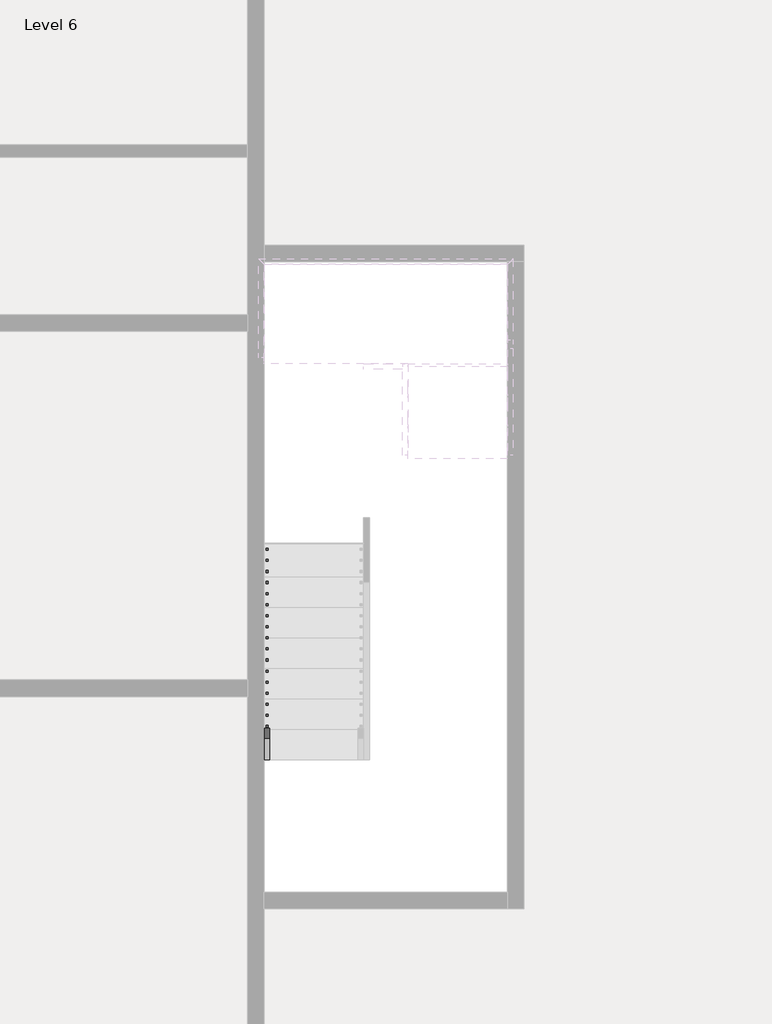
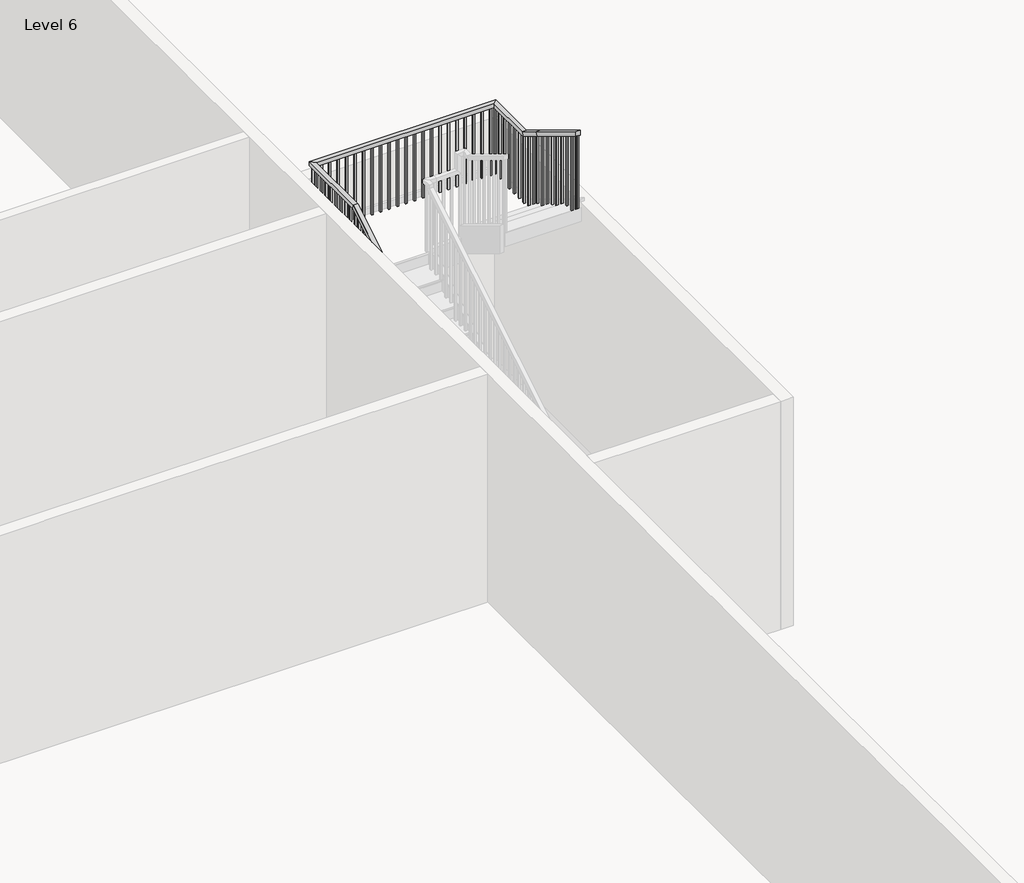
# One storey, part 6 of 8: 1 railing.
"""IFC4 building model written with IfcOpenShell, lengths in millimetres."""

from ifc_helpers import new_model, si_unit, frame, origin, place, context, project, spatial, polyline, outline, extrude, faceted_brep, element, save

model = new_model("IFC4")

# Units and contexts
model_context = context("Model", 3, world=origin())
ifc_project = project(units=[si_unit("LENGTHUNIT", "METRE", prefix="MILLI")], contexts=[model_context])

# Site, building, storey
site = spatial("IfcSite", under=ifc_project)
building = spatial("IfcBuilding", under=site)
storey = spatial("IfcBuildingStorey", under=building, Name="Level 6", Elevation=40474.6172466)

# Railing
placement = place(None, origin())
element("IfcRailing", 1, ObjectType="Handrail - Rectangular", at=placement, inside=storey, context=model_context, shape_type="SolidModel", body=[
    faceted_brep([(-3617.4415084, -23154.3851539, 41558.3505799), (-3617.4415084, -23154.3851539, 41498.9491197), (-3566.6415084, -23154.3851539, 41498.9491197), (-3566.6415084, -23154.3851539, 41558.3505799), (-3617.4415084, -19522.1851539, 43759.6839133), (-3617.4415084, -19507.9927445, 43708.8839133), (-3566.6415084, -19507.9927445, 43708.8839133), (-3566.6415084, -19522.1851539, 43759.6839133), (-3617.4415084, -18607.7851539, 43759.6839133), (-3617.4415084, -18607.7851539, 43708.8839133), (-3566.6415084, -18658.5851539, 43708.8839133), (-3566.6415084, -18658.5851539, 43759.6839133), (-1382.2415084, -18607.7851539, 43759.6839133), (-1382.2415084, -18607.7851539, 43708.8839133), (-1433.0415084, -18658.5851539, 43708.8839133), (-1433.0415084, -18658.5851539, 43759.6839133), (-1382.2415084, -19242.7851539, 43759.6839133), (-1382.2415084, -19256.9775633, 43708.8839133), (-1433.0415084, -19256.9775633, 43708.8839133), (-1433.0415084, -19242.7851539, 43759.6839133), (-1382.2415084, -19522.1851539, 43929.0172466), (-1382.2415084, -19548.5148811, 43885.5731968), (-1433.0415084, -19548.5148811, 43885.5731968), (-1433.0415084, -19522.1851539, 43929.0172466), (-1382.2415084, -20360.3851539, 44437.0172466), (-1433.0415084, -20360.3851539, 44437.0172466), (-1433.0415084, -20360.3851539, 44377.6157863), (-1382.2415084, -20360.3851539, 44377.6157863)], [[[0, 1, 2, 3]], [[1, 0, 4, 5]], [[2, 1, 5, 6]], [[3, 2, 6, 7]], [[0, 3, 7, 4]], [[5, 4, 8, 9]], [[6, 5, 9, 10]], [[7, 6, 10, 11]], [[4, 7, 11, 8]], [[9, 8, 12, 13]], [[10, 9, 13, 14]], [[11, 10, 14, 15]], [[8, 11, 15, 12]], [[13, 12, 16, 17]], [[14, 13, 17, 18]], [[15, 14, 18, 19]], [[12, 15, 19, 16]], [[17, 16, 20, 21]], [[18, 17, 21, 22]], [[19, 18, 22, 23]], [[16, 19, 23, 20]], [[24, 25, 26, 27]], [[21, 20, 24, 27]], [[22, 21, 27, 26]], [[23, 22, 26, 25]], [[20, 23, 25, 24]]]),
    extrude(outline(polyline([(-20325.4601539, 44356.4491197), (-20325.4601539, 43353.2839133), (-20344.5101539, 43353.2839133), (-20344.5101539, 44367.9945742), (-20325.4601539, 44356.4491197)])), frame((-1417.1665084, 0.0, 0.0), z_axis=(1.0, 0.0, 0.0), x_axis=(0.0, 1.0, 0.0)), (0.0, 0.0, 1.0), 19.05),
    extrude(outline(polyline([(-20223.8601539, 44294.8733621), (-20223.8601539, 43353.2839133), (-20242.9101539, 43353.2839133), (-20242.9101539, 44306.4188166), (-20223.8601539, 44294.8733621)])), frame((-1417.1665084, 0.0, 0.0), z_axis=(1.0, 0.0, 0.0), x_axis=(0.0, 1.0, 0.0)), (0.0, 0.0, 1.0), 19.05),
    extrude(outline(polyline([(-20122.2601539, 44233.2976045), (-20122.2601539, 43353.2839133), (-20141.3101539, 43353.2839133), (-20141.3101539, 44244.8430591), (-20122.2601539, 44233.2976045)])), frame((-1417.1665084, 0.0, 0.0), z_axis=(1.0, 0.0, 0.0), x_axis=(0.0, 1.0, 0.0)), (0.0, 0.0, 1.0), 19.05),
    extrude(outline(polyline([(-20020.6601539, 44171.721847), (-20020.6601539, 43183.9505799), (-20039.7101539, 43183.9505799), (-20039.7101539, 44183.2673015), (-20020.6601539, 44171.721847)])), frame((-1417.1665084, 0.0, 0.0), z_axis=(1.0, 0.0, 0.0), x_axis=(0.0, 1.0, 0.0)), (0.0, 0.0, 1.0), 19.05),
    extrude(outline(polyline([(-19919.0601539, 44110.1460894), (-19919.0601539, 43183.9505799), (-19938.1101539, 43183.9505799), (-19938.1101539, 44121.6915439), (-19919.0601539, 44110.1460894)])), frame((-1417.1665084, 0.0, 0.0), z_axis=(1.0, 0.0, 0.0), x_axis=(0.0, 1.0, 0.0)), (0.0, 0.0, 1.0), 19.05),
    extrude(outline(polyline([(-19817.4601539, 44048.5703318), (-19817.4601539, 43183.9505799), (-19836.5101539, 43183.9505799), (-19836.5101539, 44060.1157863), (-19817.4601539, 44048.5703318)])), frame((-1417.1665084, 0.0, 0.0), z_axis=(1.0, 0.0, 0.0), x_axis=(0.0, 1.0, 0.0)), (0.0, 0.0, 1.0), 19.05),
    extrude(outline(polyline([(-19715.8601539, 43986.9945742), (-19715.8601539, 43014.6172466), (-19734.9101539, 43014.6172466), (-19734.9101539, 43998.5400288), (-19715.8601539, 43986.9945742)])), frame((-1417.1665084, 0.0, 0.0), z_axis=(1.0, 0.0, 0.0), x_axis=(0.0, 1.0, 0.0)), (0.0, 0.0, 1.0), 19.05),
    extrude(outline(polyline([(-19614.2601539, 43925.4188166), (-19614.2601539, 43014.6172466), (-19633.3101539, 43014.6172466), (-19633.3101539, 43936.9642712), (-19614.2601539, 43925.4188166)])), frame((-1417.1665084, 0.0, 0.0), z_axis=(1.0, 0.0, 0.0), x_axis=(0.0, 1.0, 0.0)), (0.0, 0.0, 1.0), 19.05),
    extrude(outline(polyline([(-19436.4601539, 43817.6612409), (-19436.4601539, 42845.2839133), (-19455.5101539, 42845.2839133), (-19455.5101539, 43829.2066954), (-19436.4601539, 43817.6612409)])), frame((-1417.1665084, 0.0, 0.0), z_axis=(1.0, 0.0, 0.0), x_axis=(0.0, 1.0, 0.0)), (0.0, 0.0, 1.0), 19.05),
    extrude(outline(polyline([(-19334.8601539, 43756.0854833), (-19334.8601539, 42845.2839133), (-19353.9101539, 42845.2839133), (-19353.9101539, 43767.6309379), (-19334.8601539, 43756.0854833)])), frame((-1417.1665084, 0.0, 0.0), z_axis=(1.0, 0.0, 0.0), x_axis=(0.0, 1.0, 0.0)), (0.0, 0.0, 1.0), 19.05),
    extrude(outline(polyline([(-1398.1165084, -19233.2601539), (-1398.1165084, -19252.3101539), (-1417.1665084, -19252.3101539), (-1417.1665084, -19233.2601539), (-1398.1165084, -19233.2601539)])), frame((0.0, 0.0, 42845.2839133), z_axis=(0.0, 0.0, 1.0), x_axis=(1.0, 0.0, 0.0)), (0.0, 0.0, 1.0), 863.6),
    extrude(outline(polyline([(-1398.1165084, -19131.6601539), (-1398.1165084, -19150.7101539), (-1417.1665084, -19150.7101539), (-1417.1665084, -19131.6601539), (-1398.1165084, -19131.6601539)])), frame((0.0, 0.0, 42845.2839133), z_axis=(0.0, 0.0, 1.0), x_axis=(1.0, 0.0, 0.0)), (0.0, 0.0, 1.0), 863.6),
    extrude(outline(polyline([(-1398.1165084, -19030.0601539), (-1398.1165084, -19049.1101539), (-1417.1665084, -19049.1101539), (-1417.1665084, -19030.0601539), (-1398.1165084, -19030.0601539)])), frame((0.0, 0.0, 42845.2839133), z_axis=(0.0, 0.0, 1.0), x_axis=(1.0, 0.0, 0.0)), (0.0, 0.0, 1.0), 863.6),
    extrude(outline(polyline([(-1398.1165084, -18928.4601539), (-1398.1165084, -18947.5101539), (-1417.1665084, -18947.5101539), (-1417.1665084, -18928.4601539), (-1398.1165084, -18928.4601539)])), frame((0.0, 0.0, 42845.2839133), z_axis=(0.0, 0.0, 1.0), x_axis=(1.0, 0.0, 0.0)), (0.0, 0.0, 1.0), 863.6),
    extrude(outline(polyline([(-1398.1165084, -18826.8601539), (-1398.1165084, -18845.9101539), (-1417.1665084, -18845.9101539), (-1417.1665084, -18826.8601539), (-1398.1165084, -18826.8601539)])), frame((0.0, 0.0, 42845.2839133), z_axis=(0.0, 0.0, 1.0), x_axis=(1.0, 0.0, 0.0)), (0.0, 0.0, 1.0), 863.6),
    extrude(outline(polyline([(-1398.1165084, -18725.2601539), (-1398.1165084, -18744.3101539), (-1417.1665084, -18744.3101539), (-1417.1665084, -18725.2601539), (-1398.1165084, -18725.2601539)])), frame((0.0, 0.0, 42845.2839133), z_axis=(0.0, 0.0, 1.0), x_axis=(1.0, 0.0, 0.0)), (0.0, 0.0, 1.0), 863.6),
    extrude(outline(polyline([(-1467.9665084, -18623.6601539), (-1448.9165084, -18623.6601539), (-1448.9165084, -18642.7101539), (-1467.9665084, -18642.7101539), (-1467.9665084, -18623.6601539)])), frame((0.0, 0.0, 42845.2839133), z_axis=(0.0, 0.0, 1.0), x_axis=(1.0, 0.0, 0.0)), (0.0, 0.0, 1.0), 863.6),
    extrude(outline(polyline([(-1569.5665084, -18623.6601539), (-1550.5165084, -18623.6601539), (-1550.5165084, -18642.7101539), (-1569.5665084, -18642.7101539), (-1569.5665084, -18623.6601539)])), frame((0.0, 0.0, 42845.2839133), z_axis=(0.0, 0.0, 1.0), x_axis=(1.0, 0.0, 0.0)), (0.0, 0.0, 1.0), 863.6),
    extrude(outline(polyline([(-1671.1665084, -18623.6601539), (-1652.1165084, -18623.6601539), (-1652.1165084, -18642.7101539), (-1671.1665084, -18642.7101539), (-1671.1665084, -18623.6601539)])), frame((0.0, 0.0, 42845.2839133), z_axis=(0.0, 0.0, 1.0), x_axis=(1.0, 0.0, 0.0)), (0.0, 0.0, 1.0), 863.6),
    extrude(outline(polyline([(-1772.7665084, -18623.6601539), (-1753.7165084, -18623.6601539), (-1753.7165084, -18642.7101539), (-1772.7665084, -18642.7101539), (-1772.7665084, -18623.6601539)])), frame((0.0, 0.0, 42845.2839133), z_axis=(0.0, 0.0, 1.0), x_axis=(1.0, 0.0, 0.0)), (0.0, 0.0, 1.0), 863.6),
    extrude(outline(polyline([(-1874.3665084, -18623.6601539), (-1855.3165084, -18623.6601539), (-1855.3165084, -18642.7101539), (-1874.3665084, -18642.7101539), (-1874.3665084, -18623.6601539)])), frame((0.0, 0.0, 42845.2839133), z_axis=(0.0, 0.0, 1.0), x_axis=(1.0, 0.0, 0.0)), (0.0, 0.0, 1.0), 863.6),
    extrude(outline(polyline([(-1975.9665084, -18623.6601539), (-1956.9165084, -18623.6601539), (-1956.9165084, -18642.7101539), (-1975.9665084, -18642.7101539), (-1975.9665084, -18623.6601539)])), frame((0.0, 0.0, 42845.2839133), z_axis=(0.0, 0.0, 1.0), x_axis=(1.0, 0.0, 0.0)), (0.0, 0.0, 1.0), 863.6),
    extrude(outline(polyline([(-2077.5665084, -18623.6601539), (-2058.5165084, -18623.6601539), (-2058.5165084, -18642.7101539), (-2077.5665084, -18642.7101539), (-2077.5665084, -18623.6601539)])), frame((0.0, 0.0, 42845.2839133), z_axis=(0.0, 0.0, 1.0), x_axis=(1.0, 0.0, 0.0)), (0.0, 0.0, 1.0), 863.6),
    extrude(outline(polyline([(-2179.1665084, -18623.6601539), (-2160.1165084, -18623.6601539), (-2160.1165084, -18642.7101539), (-2179.1665084, -18642.7101539), (-2179.1665084, -18623.6601539)])), frame((0.0, 0.0, 42845.2839133), z_axis=(0.0, 0.0, 1.0), x_axis=(1.0, 0.0, 0.0)), (0.0, 0.0, 1.0), 863.6),
    extrude(outline(polyline([(-2280.7665084, -18623.6601539), (-2261.7165084, -18623.6601539), (-2261.7165084, -18642.7101539), (-2280.7665084, -18642.7101539), (-2280.7665084, -18623.6601539)])), frame((0.0, 0.0, 42845.2839133), z_axis=(0.0, 0.0, 1.0), x_axis=(1.0, 0.0, 0.0)), (0.0, 0.0, 1.0), 863.6),
    extrude(outline(polyline([(-2382.3665084, -18623.6601539), (-2363.3165084, -18623.6601539), (-2363.3165084, -18642.7101539), (-2382.3665084, -18642.7101539), (-2382.3665084, -18623.6601539)])), frame((0.0, 0.0, 42845.2839133), z_axis=(0.0, 0.0, 1.0), x_axis=(1.0, 0.0, 0.0)), (0.0, 0.0, 1.0), 863.6),
    extrude(outline(polyline([(-2483.9665084, -18623.6601539), (-2464.9165084, -18623.6601539), (-2464.9165084, -18642.7101539), (-2483.9665084, -18642.7101539), (-2483.9665084, -18623.6601539)])), frame((0.0, 0.0, 42845.2839133), z_axis=(0.0, 0.0, 1.0), x_axis=(1.0, 0.0, 0.0)), (0.0, 0.0, 1.0), 863.6),
    extrude(outline(polyline([(-2585.5665084, -18623.6601539), (-2566.5165084, -18623.6601539), (-2566.5165084, -18642.7101539), (-2585.5665084, -18642.7101539), (-2585.5665084, -18623.6601539)])), frame((0.0, 0.0, 42845.2839133), z_axis=(0.0, 0.0, 1.0), x_axis=(1.0, 0.0, 0.0)), (0.0, 0.0, 1.0), 863.6),
    extrude(outline(polyline([(-2687.1665084, -18623.6601539), (-2668.1165084, -18623.6601539), (-2668.1165084, -18642.7101539), (-2687.1665084, -18642.7101539), (-2687.1665084, -18623.6601539)])), frame((0.0, 0.0, 42845.2839133), z_axis=(0.0, 0.0, 1.0), x_axis=(1.0, 0.0, 0.0)), (0.0, 0.0, 1.0), 863.6),
    extrude(outline(polyline([(-2788.7665084, -18623.6601539), (-2769.7165084, -18623.6601539), (-2769.7165084, -18642.7101539), (-2788.7665084, -18642.7101539), (-2788.7665084, -18623.6601539)])), frame((0.0, 0.0, 42845.2839133), z_axis=(0.0, 0.0, 1.0), x_axis=(1.0, 0.0, 0.0)), (0.0, 0.0, 1.0), 863.6),
    extrude(outline(polyline([(-2890.3665084, -18623.6601539), (-2871.3165084, -18623.6601539), (-2871.3165084, -18642.7101539), (-2890.3665084, -18642.7101539), (-2890.3665084, -18623.6601539)])), frame((0.0, 0.0, 42845.2839133), z_axis=(0.0, 0.0, 1.0), x_axis=(1.0, 0.0, 0.0)), (0.0, 0.0, 1.0), 863.6),
    extrude(outline(polyline([(-2991.9665084, -18623.6601539), (-2972.9165084, -18623.6601539), (-2972.9165084, -18642.7101539), (-2991.9665084, -18642.7101539), (-2991.9665084, -18623.6601539)])), frame((0.0, 0.0, 42845.2839133), z_axis=(0.0, 0.0, 1.0), x_axis=(1.0, 0.0, 0.0)), (0.0, 0.0, 1.0), 863.6),
    extrude(outline(polyline([(-3093.5665084, -18623.6601539), (-3074.5165084, -18623.6601539), (-3074.5165084, -18642.7101539), (-3093.5665084, -18642.7101539), (-3093.5665084, -18623.6601539)])), frame((0.0, 0.0, 42845.2839133), z_axis=(0.0, 0.0, 1.0), x_axis=(1.0, 0.0, 0.0)), (0.0, 0.0, 1.0), 863.6),
    extrude(outline(polyline([(-3195.1665084, -18623.6601539), (-3176.1165084, -18623.6601539), (-3176.1165084, -18642.7101539), (-3195.1665084, -18642.7101539), (-3195.1665084, -18623.6601539)])), frame((0.0, 0.0, 42845.2839133), z_axis=(0.0, 0.0, 1.0), x_axis=(1.0, 0.0, 0.0)), (0.0, 0.0, 1.0), 863.6),
    extrude(outline(polyline([(-3296.7665084, -18623.6601539), (-3277.7165084, -18623.6601539), (-3277.7165084, -18642.7101539), (-3296.7665084, -18642.7101539), (-3296.7665084, -18623.6601539)])), frame((0.0, 0.0, 42845.2839133), z_axis=(0.0, 0.0, 1.0), x_axis=(1.0, 0.0, 0.0)), (0.0, 0.0, 1.0), 863.6),
    extrude(outline(polyline([(-3398.3665084, -18623.6601539), (-3379.3165084, -18623.6601539), (-3379.3165084, -18642.7101539), (-3398.3665084, -18642.7101539), (-3398.3665084, -18623.6601539)])), frame((0.0, 0.0, 42845.2839133), z_axis=(0.0, 0.0, 1.0), x_axis=(1.0, 0.0, 0.0)), (0.0, 0.0, 1.0), 863.6),
    extrude(outline(polyline([(-3499.9665084, -18623.6601539), (-3480.9165084, -18623.6601539), (-3480.9165084, -18642.7101539), (-3499.9665084, -18642.7101539), (-3499.9665084, -18623.6601539)])), frame((0.0, 0.0, 42845.2839133), z_axis=(0.0, 0.0, 1.0), x_axis=(1.0, 0.0, 0.0)), (0.0, 0.0, 1.0), 863.6),
    extrude(outline(polyline([(-3601.5665084, -18718.9101539), (-3601.5665084, -18699.8601539), (-3582.5165084, -18699.8601539), (-3582.5165084, -18718.9101539), (-3601.5665084, -18718.9101539)])), frame((0.0, 0.0, 42845.2839133), z_axis=(0.0, 0.0, 1.0), x_axis=(1.0, 0.0, 0.0)), (0.0, 0.0, 1.0), 863.6),
    extrude(outline(polyline([(-3601.5665084, -18820.5101539), (-3601.5665084, -18801.4601539), (-3582.5165084, -18801.4601539), (-3582.5165084, -18820.5101539), (-3601.5665084, -18820.5101539)])), frame((0.0, 0.0, 42845.2839133), z_axis=(0.0, 0.0, 1.0), x_axis=(1.0, 0.0, 0.0)), (0.0, 0.0, 1.0), 863.6),
    extrude(outline(polyline([(-3601.5665084, -18922.1101539), (-3601.5665084, -18903.0601539), (-3582.5165084, -18903.0601539), (-3582.5165084, -18922.1101539), (-3601.5665084, -18922.1101539)])), frame((0.0, 0.0, 42845.2839133), z_axis=(0.0, 0.0, 1.0), x_axis=(1.0, 0.0, 0.0)), (0.0, 0.0, 1.0), 863.6),
    extrude(outline(polyline([(-3601.5665084, -19023.7101539), (-3601.5665084, -19004.6601539), (-3582.5165084, -19004.6601539), (-3582.5165084, -19023.7101539), (-3601.5665084, -19023.7101539)])), frame((0.0, 0.0, 42845.2839133), z_axis=(0.0, 0.0, 1.0), x_axis=(1.0, 0.0, 0.0)), (0.0, 0.0, 1.0), 863.6),
    extrude(outline(polyline([(-3601.5665084, -19125.3101539), (-3601.5665084, -19106.2601539), (-3582.5165084, -19106.2601539), (-3582.5165084, -19125.3101539), (-3601.5665084, -19125.3101539)])), frame((0.0, 0.0, 42845.2839133), z_axis=(0.0, 0.0, 1.0), x_axis=(1.0, 0.0, 0.0)), (0.0, 0.0, 1.0), 863.6),
    extrude(outline(polyline([(-3601.5665084, -19226.9101539), (-3601.5665084, -19207.8601539), (-3582.5165084, -19207.8601539), (-3582.5165084, -19226.9101539), (-3601.5665084, -19226.9101539)])), frame((0.0, 0.0, 42845.2839133), z_axis=(0.0, 0.0, 1.0), x_axis=(1.0, 0.0, 0.0)), (0.0, 0.0, 1.0), 863.6),
    extrude(outline(polyline([(-3601.5665084, -19328.5101539), (-3601.5665084, -19309.4601539), (-3582.5165084, -19309.4601539), (-3582.5165084, -19328.5101539), (-3601.5665084, -19328.5101539)])), frame((0.0, 0.0, 42845.2839133), z_axis=(0.0, 0.0, 1.0), x_axis=(1.0, 0.0, 0.0)), (0.0, 0.0, 1.0), 863.6),
    extrude(outline(polyline([(-3601.5665084, -19430.1101539), (-3601.5665084, -19411.0601539), (-3582.5165084, -19411.0601539), (-3582.5165084, -19430.1101539), (-3601.5665084, -19430.1101539)])), frame((0.0, 0.0, 42845.2839133), z_axis=(0.0, 0.0, 1.0), x_axis=(1.0, 0.0, 0.0)), (0.0, 0.0, 1.0), 863.6),
    extrude(outline(polyline([(-19588.8601539, 43659.8733621), (-19588.8601539, 42675.9505799), (-19607.9101539, 42675.9505799), (-19607.9101539, 43648.3279076), (-19588.8601539, 43659.8733621)])), frame((-3601.5665084, 0.0, 0.0), z_axis=(1.0, 0.0, 0.0), x_axis=(0.0, 1.0, 0.0)), (0.0, 0.0, 1.0), 19.05),
    extrude(outline(polyline([(-19690.4601539, 43598.2976045), (-19690.4601539, 42675.9505799), (-19709.5101539, 42675.9505799), (-19709.5101539, 43586.75215), (-19690.4601539, 43598.2976045)])), frame((-3601.5665084, 0.0, 0.0), z_axis=(1.0, 0.0, 0.0), x_axis=(0.0, 1.0, 0.0)), (0.0, 0.0, 1.0), 19.05),
    extrude(outline(polyline([(-19792.0601539, 43536.721847), (-19792.0601539, 42675.9505799), (-19811.1101539, 42675.9505799), (-19811.1101539, 43525.1763924), (-19792.0601539, 43536.721847)])), frame((-3601.5665084, 0.0, 0.0), z_axis=(1.0, 0.0, 0.0), x_axis=(0.0, 1.0, 0.0)), (0.0, 0.0, 1.0), 19.05),
    extrude(outline(polyline([(-19893.6601539, 43475.1460894), (-19893.6601539, 42506.6172466), (-19912.7101539, 42506.6172466), (-19912.7101539, 43463.6006348), (-19893.6601539, 43475.1460894)])), frame((-3601.5665084, 0.0, 0.0), z_axis=(1.0, 0.0, 0.0), x_axis=(0.0, 1.0, 0.0)), (0.0, 0.0, 1.0), 19.05),
    extrude(outline(polyline([(-19995.2601539, 43413.5703318), (-19995.2601539, 42506.6172466), (-20014.3101539, 42506.6172466), (-20014.3101539, 43402.0248773), (-19995.2601539, 43413.5703318)])), frame((-3601.5665084, 0.0, 0.0), z_axis=(1.0, 0.0, 0.0), x_axis=(0.0, 1.0, 0.0)), (0.0, 0.0, 1.0), 19.05),
    extrude(outline(polyline([(-20096.8601539, 43351.9945742), (-20096.8601539, 42337.2839133), (-20115.9101539, 42337.2839133), (-20115.9101539, 43340.4491197), (-20096.8601539, 43351.9945742)])), frame((-3601.5665084, 0.0, 0.0), z_axis=(1.0, 0.0, 0.0), x_axis=(0.0, 1.0, 0.0)), (0.0, 0.0, 1.0), 19.05),
    extrude(outline(polyline([(-20198.4601539, 43290.4188166), (-20198.4601539, 42337.2839133), (-20217.5101539, 42337.2839133), (-20217.5101539, 43278.8733621), (-20198.4601539, 43290.4188166)])), frame((-3601.5665084, 0.0, 0.0), z_axis=(1.0, 0.0, 0.0), x_axis=(0.0, 1.0, 0.0)), (0.0, 0.0, 1.0), 19.05),
    extrude(outline(polyline([(-20300.0601539, 43228.8430591), (-20300.0601539, 42337.2839133), (-20319.1101539, 42337.2839133), (-20319.1101539, 43217.2976045), (-20300.0601539, 43228.8430591)])), frame((-3601.5665084, 0.0, 0.0), z_axis=(1.0, 0.0, 0.0), x_axis=(0.0, 1.0, 0.0)), (0.0, 0.0, 1.0), 19.05),
    extrude(outline(polyline([(-20401.6601539, 43167.2673015), (-20401.6601539, 42167.9505799), (-20420.7101539, 42167.9505799), (-20420.7101539, 43155.721847), (-20401.6601539, 43167.2673015)])), frame((-3601.5665084, 0.0, 0.0), z_axis=(1.0, 0.0, 0.0), x_axis=(0.0, 1.0, 0.0)), (0.0, 0.0, 1.0), 19.05),
    extrude(outline(polyline([(-20503.2601539, 43105.6915439), (-20503.2601539, 42167.9505799), (-20522.3101539, 42167.9505799), (-20522.3101539, 43094.1460894), (-20503.2601539, 43105.6915439)])), frame((-3601.5665084, 0.0, 0.0), z_axis=(1.0, 0.0, 0.0), x_axis=(0.0, 1.0, 0.0)), (0.0, 0.0, 1.0), 19.05),
    extrude(outline(polyline([(-20604.8601539, 43044.1157863), (-20604.8601539, 42167.9505799), (-20623.9101539, 42167.9505799), (-20623.9101539, 43032.5703318), (-20604.8601539, 43044.1157863)])), frame((-3601.5665084, 0.0, 0.0), z_axis=(1.0, 0.0, 0.0), x_axis=(0.0, 1.0, 0.0)), (0.0, 0.0, 1.0), 19.05),
    extrude(outline(polyline([(-20706.4601539, 42982.5400288), (-20706.4601539, 41998.6172466), (-20725.5101539, 41998.6172466), (-20725.5101539, 42970.9945742), (-20706.4601539, 42982.5400288)])), frame((-3601.5665084, 0.0, 0.0), z_axis=(1.0, 0.0, 0.0), x_axis=(0.0, 1.0, 0.0)), (0.0, 0.0, 1.0), 19.05),
    extrude(outline(polyline([(-20808.0601539, 42920.9642712), (-20808.0601539, 41998.6172466), (-20827.1101539, 41998.6172466), (-20827.1101539, 42909.4188166), (-20808.0601539, 42920.9642712)])), frame((-3601.5665084, 0.0, 0.0), z_axis=(1.0, 0.0, 0.0), x_axis=(0.0, 1.0, 0.0)), (0.0, 0.0, 1.0), 19.05),
    extrude(outline(polyline([(-20909.6601539, 42859.3885136), (-20909.6601539, 41998.6172466), (-20928.7101539, 41998.6172466), (-20928.7101539, 42847.8430591), (-20909.6601539, 42859.3885136)])), frame((-3601.5665084, 0.0, 0.0), z_axis=(1.0, 0.0, 0.0), x_axis=(0.0, 1.0, 0.0)), (0.0, 0.0, 1.0), 19.05),
    extrude(outline(polyline([(-21011.2601539, 42797.812756), (-21011.2601539, 41829.2839133), (-21030.3101539, 41829.2839133), (-21030.3101539, 42786.2673015), (-21011.2601539, 42797.812756)])), frame((-3601.5665084, 0.0, 0.0), z_axis=(1.0, 0.0, 0.0), x_axis=(0.0, 1.0, 0.0)), (0.0, 0.0, 1.0), 19.05),
    extrude(outline(polyline([(-21112.8601539, 42736.2369985), (-21112.8601539, 41829.2839133), (-21131.9101539, 41829.2839133), (-21131.9101539, 42724.6915439), (-21112.8601539, 42736.2369985)])), frame((-3601.5665084, 0.0, 0.0), z_axis=(1.0, 0.0, 0.0), x_axis=(0.0, 1.0, 0.0)), (0.0, 0.0, 1.0), 19.05),
    extrude(outline(polyline([(-21214.4601539, 42674.6612409), (-21214.4601539, 41659.9505799), (-21233.5101539, 41659.9505799), (-21233.5101539, 42663.1157863), (-21214.4601539, 42674.6612409)])), frame((-3601.5665084, 0.0, 0.0), z_axis=(1.0, 0.0, 0.0), x_axis=(0.0, 1.0, 0.0)), (0.0, 0.0, 1.0), 19.05),
    extrude(outline(polyline([(-21316.0601539, 42613.0854833), (-21316.0601539, 41659.9505799), (-21335.1101539, 41659.9505799), (-21335.1101539, 42601.5400288), (-21316.0601539, 42613.0854833)])), frame((-3601.5665084, 0.0, 0.0), z_axis=(1.0, 0.0, 0.0), x_axis=(0.0, 1.0, 0.0)), (0.0, 0.0, 1.0), 19.05),
    extrude(outline(polyline([(-21417.6601539, 42551.5097257), (-21417.6601539, 41659.9505799), (-21436.7101539, 41659.9505799), (-21436.7101539, 42539.9642712), (-21417.6601539, 42551.5097257)])), frame((-3601.5665084, 0.0, 0.0), z_axis=(1.0, 0.0, 0.0), x_axis=(0.0, 1.0, 0.0)), (0.0, 0.0, 1.0), 19.05),
    extrude(outline(polyline([(-21519.2601539, 42489.9339682), (-21519.2601539, 41490.6172466), (-21538.3101539, 41490.6172466), (-21538.3101539, 42478.3885136), (-21519.2601539, 42489.9339682)])), frame((-3601.5665084, 0.0, 0.0), z_axis=(1.0, 0.0, 0.0), x_axis=(0.0, 1.0, 0.0)), (0.0, 0.0, 1.0), 19.05),
    extrude(outline(polyline([(-21620.8601539, 42428.3582106), (-21620.8601539, 41490.6172466), (-21639.9101539, 41490.6172466), (-21639.9101539, 42416.812756), (-21620.8601539, 42428.3582106)])), frame((-3601.5665084, 0.0, 0.0), z_axis=(1.0, 0.0, 0.0), x_axis=(0.0, 1.0, 0.0)), (0.0, 0.0, 1.0), 19.05),
    extrude(outline(polyline([(-21722.4601539, 42366.782453), (-21722.4601539, 41490.6172466), (-21741.5101539, 41490.6172466), (-21741.5101539, 42355.2369985), (-21722.4601539, 42366.782453)])), frame((-3601.5665084, 0.0, 0.0), z_axis=(1.0, 0.0, 0.0), x_axis=(0.0, 1.0, 0.0)), (0.0, 0.0, 1.0), 19.05),
    extrude(outline(polyline([(-21824.0601539, 42305.2066954), (-21824.0601539, 41321.2839133), (-21843.1101539, 41321.2839133), (-21843.1101539, 42293.6612409), (-21824.0601539, 42305.2066954)])), frame((-3601.5665084, 0.0, 0.0), z_axis=(1.0, 0.0, 0.0), x_axis=(0.0, 1.0, 0.0)), (0.0, 0.0, 1.0), 19.05),
    extrude(outline(polyline([(-21925.6601539, 42243.6309379), (-21925.6601539, 41321.2839133), (-21944.7101539, 41321.2839133), (-21944.7101539, 42232.0854833), (-21925.6601539, 42243.6309379)])), frame((-3601.5665084, 0.0, 0.0), z_axis=(1.0, 0.0, 0.0), x_axis=(0.0, 1.0, 0.0)), (0.0, 0.0, 1.0), 19.05),
    extrude(outline(polyline([(-22027.2601539, 42182.0551803), (-22027.2601539, 41321.2839133), (-22046.3101539, 41321.2839133), (-22046.3101539, 42170.5097257), (-22027.2601539, 42182.0551803)])), frame((-3601.5665084, 0.0, 0.0), z_axis=(1.0, 0.0, 0.0), x_axis=(0.0, 1.0, 0.0)), (0.0, 0.0, 1.0), 19.05),
    extrude(outline(polyline([(-22128.8601539, 42120.4794227), (-22128.8601539, 41151.9505799), (-22147.9101539, 41151.9505799), (-22147.9101539, 42108.9339682), (-22128.8601539, 42120.4794227)])), frame((-3601.5665084, 0.0, 0.0), z_axis=(1.0, 0.0, 0.0), x_axis=(0.0, 1.0, 0.0)), (0.0, 0.0, 1.0), 19.05),
    extrude(outline(polyline([(-22230.4601539, 42058.9036651), (-22230.4601539, 41151.9505799), (-22249.5101539, 41151.9505799), (-22249.5101539, 42047.3582106), (-22230.4601539, 42058.9036651)])), frame((-3601.5665084, 0.0, 0.0), z_axis=(1.0, 0.0, 0.0), x_axis=(0.0, 1.0, 0.0)), (0.0, 0.0, 1.0), 19.05),
    extrude(outline(polyline([(-22332.0601539, 41997.3279076), (-22332.0601539, 40982.6172466), (-22351.1101539, 40982.6172466), (-22351.1101539, 41985.782453), (-22332.0601539, 41997.3279076)])), frame((-3601.5665084, 0.0, 0.0), z_axis=(1.0, 0.0, 0.0), x_axis=(0.0, 1.0, 0.0)), (0.0, 0.0, 1.0), 19.05),
    extrude(outline(polyline([(-22433.6601539, 41935.75215), (-22433.6601539, 40982.6172466), (-22452.7101539, 40982.6172466), (-22452.7101539, 41924.2066954), (-22433.6601539, 41935.75215)])), frame((-3601.5665084, 0.0, 0.0), z_axis=(1.0, 0.0, 0.0), x_axis=(0.0, 1.0, 0.0)), (0.0, 0.0, 1.0), 19.05),
    extrude(outline(polyline([(-22535.2601539, 41874.1763924), (-22535.2601539, 40982.6172466), (-22554.3101539, 40982.6172466), (-22554.3101539, 41862.6309379), (-22535.2601539, 41874.1763924)])), frame((-3601.5665084, 0.0, 0.0), z_axis=(1.0, 0.0, 0.0), x_axis=(0.0, 1.0, 0.0)), (0.0, 0.0, 1.0), 19.05),
    extrude(outline(polyline([(-22636.8601539, 41812.6006348), (-22636.8601539, 40813.2839133), (-22655.9101539, 40813.2839133), (-22655.9101539, 41801.0551803), (-22636.8601539, 41812.6006348)])), frame((-3601.5665084, 0.0, 0.0), z_axis=(1.0, 0.0, 0.0), x_axis=(0.0, 1.0, 0.0)), (0.0, 0.0, 1.0), 19.05),
    extrude(outline(polyline([(-22738.4601539, 41751.0248773), (-22738.4601539, 40813.2839133), (-22757.5101539, 40813.2839133), (-22757.5101539, 41739.4794227), (-22738.4601539, 41751.0248773)])), frame((-3601.5665084, 0.0, 0.0), z_axis=(1.0, 0.0, 0.0), x_axis=(0.0, 1.0, 0.0)), (0.0, 0.0, 1.0), 19.05),
    extrude(outline(polyline([(-22840.0601539, 41689.4491197), (-22840.0601539, 40813.2839133), (-22859.1101539, 40813.2839133), (-22859.1101539, 41677.9036651), (-22840.0601539, 41689.4491197)])), frame((-3601.5665084, 0.0, 0.0), z_axis=(1.0, 0.0, 0.0), x_axis=(0.0, 1.0, 0.0)), (0.0, 0.0, 1.0), 19.05),
    extrude(outline(polyline([(-22941.6601539, 41627.8733621), (-22941.6601539, 40643.9505799), (-22960.7101539, 40643.9505799), (-22960.7101539, 41616.3279076), (-22941.6601539, 41627.8733621)])), frame((-3601.5665084, 0.0, 0.0), z_axis=(1.0, 0.0, 0.0), x_axis=(0.0, 1.0, 0.0)), (0.0, 0.0, 1.0), 19.05),
    extrude(outline(polyline([(-23043.2601539, 41566.2976045), (-23043.2601539, 40643.9505799), (-23062.3101539, 40643.9505799), (-23062.3101539, 41554.75215), (-23043.2601539, 41566.2976045)])), frame((-3601.5665084, 0.0, 0.0), z_axis=(1.0, 0.0, 0.0), x_axis=(0.0, 1.0, 0.0)), (0.0, 0.0, 1.0), 19.05),
    extrude(outline(polyline([(-19512.6601539, 43863.8430591), (-19512.6601539, 42845.2839133), (-19531.7101539, 42845.2839133), (-19531.7101539, 43875.3885136), (-19512.6601539, 43863.8430591)])), frame((-1417.1665084, 0.0, 0.0), z_axis=(1.0, 0.0, 0.0), x_axis=(0.0, 1.0, 0.0)), (0.0, 0.0, 1.0), 19.05),
    extrude(outline(polyline([(-1417.1665084, -18623.6601539), (-1398.1165084, -18623.6601539), (-1398.1165084, -18642.7101539), (-1417.1665084, -18642.7101539), (-1417.1665084, -18623.6601539)])), frame((0.0, 0.0, 42845.2839133), z_axis=(0.0, 0.0, 1.0), x_axis=(1.0, 0.0, 0.0)), (0.0, 0.0, 1.0), 863.6),
    extrude(outline(polyline([(-3601.5665084, -18642.7101539), (-3601.5665084, -18623.6601539), (-3582.5165084, -18623.6601539), (-3582.5165084, -18642.7101539), (-3601.5665084, -18642.7101539)])), frame((0.0, 0.0, 42845.2839133), z_axis=(0.0, 0.0, 1.0), x_axis=(1.0, 0.0, 0.0)), (0.0, 0.0, 1.0), 863.6),
    extrude(outline(polyline([(-19512.6601539, 43706.0551803), (-19512.6601539, 42845.2839133), (-19531.7101539, 42845.2839133), (-19531.7101539, 43694.5097257), (-19512.6601539, 43706.0551803)])), frame((-3601.5665084, 0.0, 0.0), z_axis=(1.0, 0.0, 0.0), x_axis=(0.0, 1.0, 0.0)), (0.0, 0.0, 1.0), 19.05),
    extrude(outline(polyline([(-20341.3351539, 44366.0703318), (-20341.3351539, 43353.2839133), (-20360.3851539, 43353.2839133), (-20360.3851539, 44377.6157863), (-20341.3351539, 44366.0703318)])), frame((-1417.1665084, 0.0, 0.0), z_axis=(1.0, 0.0, 0.0), x_axis=(0.0, 1.0, 0.0)), (0.0, 0.0, 1.0), 19.05),
    extrude(outline(polyline([(-23135.3351539, 41510.4945742), (-23135.3351539, 40643.9505799), (-23154.3851539, 40643.9505799), (-23154.3851539, 41498.9491197), (-23135.3351539, 41510.4945742)])), frame((-3601.5665084, 0.0, 0.0), z_axis=(1.0, 0.0, 0.0), x_axis=(0.0, 1.0, 0.0)), (0.0, 0.0, 1.0), 19.05),
])

save(model, "model.ifc")

# Revit data of these elements
# Type "Handrail - Rectangular"
#   Assembly Code = "C2010400"
#   built-in parameter 1008612 = 0.0416667 (stored number, unit not read)
#   built-in parameter 1008611 = 0.0416667 (stored number, unit not read)
#   built-in parameter 1008609 = 0.333333 (stored number, unit not read)
#   built-in parameter 1008604 = 0.166667 (stored number, unit not read)
#   built-in parameter 1008603 = 0.166667 (stored number, unit not read)
#   Railing Height = 3' - 0"
#   built-in parameter 1008630 = 2
#   built-in parameter 1008610 = 2
#   built-in parameter 1008618 = Baluster - Square : 3/4"
# Element 1 (IfcRailing, "Handrail - Rectangular")
#   Phase Created = New Construction
